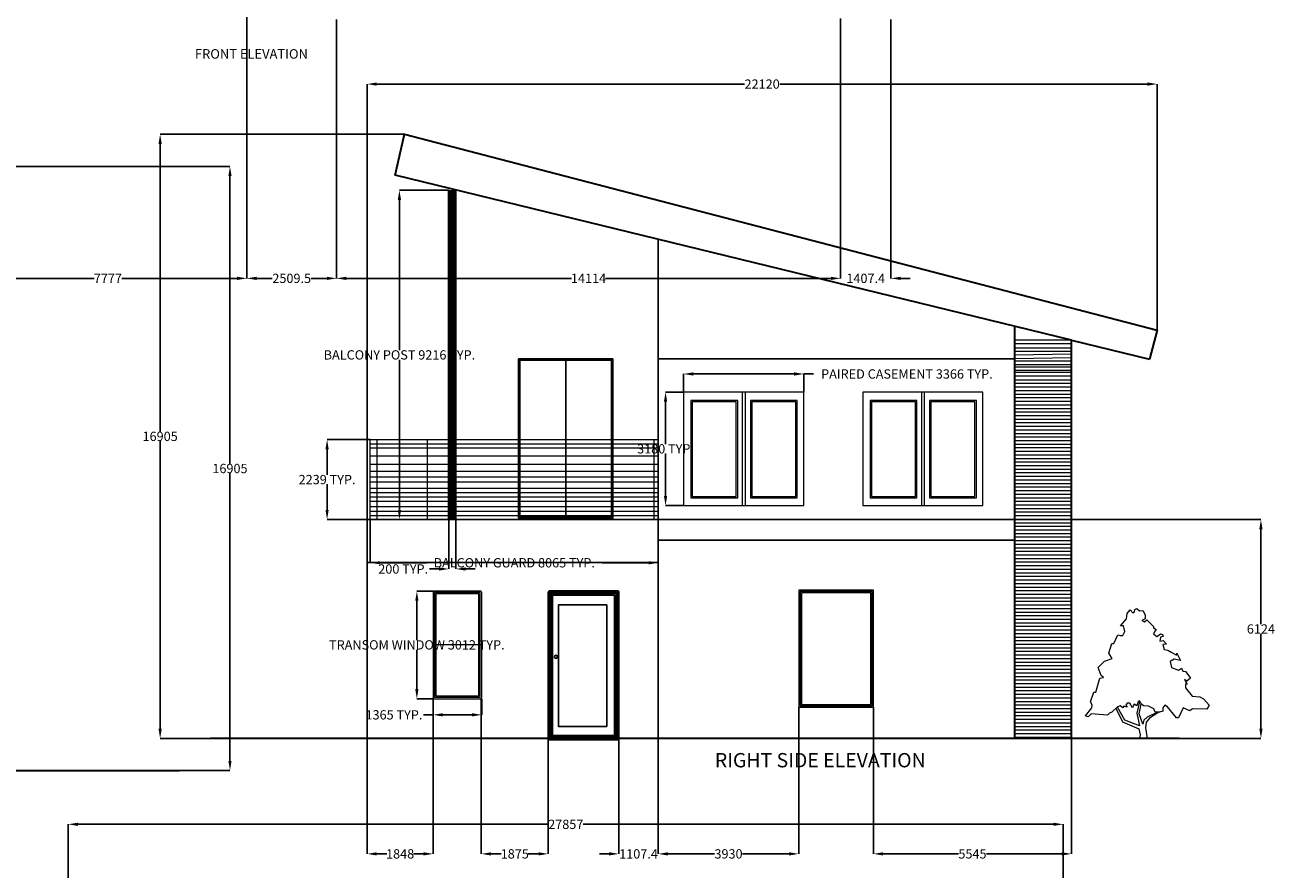
# Model space of a CAD drawing. Units: millimetres. Extents: x 23 to 3809233, y 4 to 290343.
# Tile 6 of 8: x 1915648 to 1950647, y 149481 to 173128. Entities that reach past the tile are written whole.
import ezdxf

# ---------------------------------------------------------------- set-up
doc = ezdxf.new("R2010")
doc.units = ezdxf.units.MM
doc.header["$MEASUREMENT"] = 0
for name, color, linetype, lineweight in [('A-ANNO-DIMS', 2, 'Continuous', 18), ('A-ANNO-TEXT', 7, 'Continuous', 25), ('A-COLS', 7, 'Continuous', 35), ('A-DOOR', 3, 'Continuous', 25), ('A-ELEV', 7, 'Continuous', 25), ('A-ELEV-GRND', 7, 'Continuous', 30), ('A-FLOR-RAIL', 8, 'Continuous', 18), ('A-GLAZ', 4, 'Continuous', 18), ('A-ROOF', 7, 'Continuous', 35), ('A-WALL-PATT', 252, 'Continuous', 13), ('L-PLNT', 94, 'Continuous', 13)]:
    doc.layers.add(name, color=color, linetype=linetype, lineweight=lineweight)
doc.styles.get("Standard").update_dxf_attribs({"font": 'arial.ttf'})
doc.dimstyles.get("Standard").update_dxf_attribs({"dimtxt": 260.18, "dimasz": 270.18, "dimexe": 0.18, "dimexo": 0.0625, "dimgap": 0.09, "dimtad": 0, "dimtih": 1, "dimtoh": 1, "dimdec": 0, "dimzin": 0, "dimdsep": 46, "dimtxsty": 'Standard', "dimcen": 0.09, "dimadec": 0, "dimazin": 0, "dimtfac": 1, "dimtdec": 0, "dimtofl": 0, "dimtmove": 0, "dimatfit": 3, "dimfxl": 1, "dimtolj": 1, "dimtzin": 0, "dimarcsym": 0})

# ---------------------------------------------------------------- blocks, each defined once
blk = doc.blocks.new('*U4')
for points in [[(22.0124, 137.721), (18.5475, 141.5624), (15.5282, 138.2446), (13.8028, 139.3505), (13.3714, 142.1153), (11.2148, 143.2214), (8.1954, 140.4564), (4.7447, 141.0094), (2.1567, 136.0326), (2.1567, 131.6088), (5.6074, 129.9499), (3.0193, 128.2909), (0.4313, 130.5029), (-6.9015, 123.3141), (-6.9015, 121.6552), (-9.9208, 119.9963), (-9.0581, 118.3373), (-6.9015, 115.0195), (-10.7835, 112.2546), (-14.6656, 115.0195), (-16.8222, 114.4665), (-17.6849, 112.2546), (-14.6656, 111.7016), (-14.2342, 107.2778), (-17.6065, 107.8307), (-21.5669, 103.9599), (-17.2536, 103.4069), (-18.9789, 97.8771), (-22.8609, 97.3241), (-27.1743, 94.5593), (-32.3504, 91.7944), (-32.7817, 94.0063), (-36.6638, 85.7116), (-29.7624, 87.3705), (-25.449, 84.6056), (-26.743, 77.9699), (-34.507, 75.205), (-37.9578, 77.4169), (-39.2518, 74.099), (-42.2711, 73.5461), (-44.8592, 70.2282), (-47.8786, 66.3574), (-43.9965, 63.0395), (-41.4085, 64.6985), (-44.3346, 59.8898), (-42.2089, 60.1377), (-42.5159, 55.7849), (-49.6039, 46.4502), (-58.2307, 45.8972), (-62.1127, 43.6853), (-68.5828, 36.4966), (-65.9947, 32.0727), (-50.0352, 32.6257), (-47.0159, 30.4138), (-39.6831, 33.7317), (-34.507, 22.6721), (-32.3504, 22.6721), (-22.4296, 34.8376), (-19.4102, 36.4966), (-17.2536, 33.7317), (-17.2536, 29.8608), (-13.8028, 28.7549), (-9.0581, 28.7549), (-7.3328, 32.6257), (-1.7254, 35.3906), (3.8821, 35.9436), (6.4701, 38.1555), (6.9014, 38.7085), (8.1954, 41.4734), (9.9208, 40.3674), (11.2148, 35.9436), (14.2341, 37.6025), (15.0968, 36.4966), (15.9595, 33.7317), (18.9789, 38.7085), (21.9982, 38.7085), (23.2922, 36.4966), (21.9982, 34.2847), (25.4489, 35.3906), (26.743, 33.7317), (29.7623, 35.9436), (32.7817, 34.8376), (38.8204, 28.7549), (41.4084, 27.6489), (43.5651, 25.437), (61.6813, 27.0959), (65.132, 23.7781), (67.7201, 24.884), (60.8186, 33.7317), (60.3873, 37.0495), (62.544, 40.3674), (58.662, 50.874), (56.5053, 50.874), (52.1919, 66.3574), (47.8785, 66.9103), (50.4665, 69.1222), (53.9172, 77.9699), (47.0158, 85.1586), (38.3891, 87.9235), (42.2711, 94.0063)], [(42.2711, 94.0063), (38.8204, 104.5129), (36.6637, 104.5129), (32.3503, 113.9135), (29.7623, 113.3605), (26.743, 113.3605), (24.5862, 117.7844), (25.8802, 123.8671), (29.331, 123.8671), (22.8609, 131.6088), (21.9982, 137.6916)], [(-12.9401, 28.7549), (-2.588, 22.1191), (0.8626, 17.6953), (1.7253, 11.6125), (0, 0)], [(-9.9208, 28.2019), (0, 23.2251), (3.4507, 19.9072), (4.7447, 15.4834), (8.6267, 27.0959), (6.4701, 37.6025)], [(34.5071, 33.1787), (27.1743, 18.2483), (9.0581, 10.5066), (7.7641, 3.8708), (8.1954, 0)], [(8.1954, 40.3674), (11.2148, 27.6489), (8.1954, 13.8245), (24.5862, 19.9072), (32.7817, 34.2847)]]:
    blk.add_lwpolyline(points)
blk = doc.blocks.new('SIDE-ENTRY-DOOR-ELEV')
for points in [[(0, 4129, -0.414214), (43, 4172), (1935, 4172, -0.414214), (1978, 4129), (1978, 43, -0.414214), (1935, 0), (43, 0, -0.414214), (0, 43)], [(40, 4129, -0.414214), (43, 4132), (1935, 4132, -0.414214), (1938, 4129), (1938, 43, -0.414214), (1935, 40), (43, 40, -0.414214), (40, 43)], [(337, 3772, -0.414214), (340, 3775), (1691, 3775, -0.414214), (1694, 3772), (1694, 380, -0.414214), (1691, 377), (340, 377, -0.414214), (337, 380)]]:
    blk.add_lwpolyline(points, format="xyb", close=True)
for points in [[(80, 4092), (1898, 4092), (1898, 80), (80, 80)], [(120, 4052), (1858, 4052), (1858, 120), (120, 120)]]:
    blk.add_lwpolyline(points, close=True)
blk.add_circle((1762, 2322), 43.3)
blk = doc.blocks.new('FIXED-WINDOW-ELEV')
blk.add_lwpolyline([(0, 3279, -0.414214), (3, 3282), (2093, 3282, -0.414214), (2096, 3279), (2096, 3, -0.414214), (2093, 0), (3, 0, -0.414214), (0, 3)], format="xyb", close=True)
for points in [[(40, 3242), (2056, 3242), (2056, 40), (40, 40)], [(80, 3202), (2016, 3202), (2016, 80), (80, 80)]]:
    blk.add_lwpolyline(points, close=True)
blk = doc.blocks.new('TRANSOM-WINDOW-ELEV')
blk.add_line((0, 1506), (1365, 1506))
for points in [[(0, 2969, -0.414214), (43, 3012), (1322, 3012, -0.414214), (1365, 2969), (1365, 43, -0.414214), (1322, 0), (43, 0, -0.414214), (0, 43)], [(40, 2969, -0.414214), (43, 2972), (1322, 2972, -0.414214), (1325, 2969), (1325, 43, -0.414214), (1322, 40), (43, 40, -0.414214), (40, 43)]]:
    blk.add_lwpolyline(points, format="xyb", close=True)
blk.add_lwpolyline([(80, 2932), (1285, 2932), (1285, 80), (80, 80)], close=True)
blk = doc.blocks.new('BALCONY-GUARD-ELEV')
for p, q in [((8065, 2239), (0, 2239)), ((0, 2109), (8065, 2109)), ((129, 2239), (129, 0)), ((6472, 2239), (6472, 0)), ((7879, 2239), (7879, 0)), ((8065, 0), (8065, 2239)), ((0, 1995), (8065, 1995)), ((0, 1772), (8065, 1772)), ((0, 1540), (8065, 1540)), ((0, 1341), (8065, 1341)), ((0, 1187), (8065, 1187)), ((0, 1045), (8065, 1045)), ((0, 866), (8065, 866)), ((0, 745), (8065, 745)), ((0, 622), (8065, 622)), ((0, 507), (8065, 507)), ((0, 360), (8065, 360)), ((8065, 360), (8065, 360)), ((0, 225), (8065, 225)), ((0, 103), (8065, 103))]:
    blk.add_line(p, q)
blk = doc.blocks.new('PAIRED-CASEMENT-ELEV')
for p, q in [((1643, 3180), (1643, 0)), ((1723, 3180), (1723, 0))]:
    blk.add_line(p, q)
for points in [[(3366, 3177, 0.414214), (3363, 3180), (3, 3180, 0.414214), (0, 3177), (0, 3, 0.414214), (3, 0), (3363, 0, 0.414214), (3366, 3)], [(1515, 2942, 0.414214), (1512, 2945), (206, 2945, 0.414214), (203, 2942), (203, 222, 0.414214), (206, 219), (1512, 219, 0.414214), (1515, 222)], [(3181, 2942, 0.414214), (3178, 2945), (1873, 2945, 0.414214), (1870, 2942), (1870, 222, 0.414214), (1873, 219), (3178, 219, 0.414214), (3181, 222)]]:
    blk.add_lwpolyline(points, format="xyb", close=True)
for points in [[(1475, 2905), (243, 2905), (243, 259), (1475, 259)], [(3141, 2905), (1910, 2905), (1910, 259), (3141, 259)]]:
    blk.add_lwpolyline(points, close=True)
blk = doc.blocks.new('ROOF-FASCIA-SIDE-ELEV')
for p, q in [((21076, 6297), (0, 817)), ((21331, 5154), (21076, 6297)), ((2399, 534), (21331, 5154)), ((0, 817), (212, 0)), ((2399, 534), (212, 0))]:
    blk.add_line(p, q)
blk = doc.blocks.new('BALCONY-SUPPORT-ELEV')
for p, q in [((0, 0), (0, 9216)), ((40, 0), (40, 9216)), ((80, 0), (80, 9216)), ((120, 0), (120, 9216)), ((120, 0), (120, 9216)), ((160, 0), (160, 9216)), ((200, 0), (200, 9216))]:
    blk.add_line(p, q)
blk = doc.blocks.new('BALCONY-GLAZED-DOOR-ELEV')
for p, q in [((0, 4461), (2642, 4461)), ((0, 4421), (2642, 4421)), ((1321, 4461), (1321, 0))]:
    blk.add_line(p, q)
for points in [[(0, 4461), (0, 0), (2642, 0), (2642, 4461)], [(40, 4461), (40, 40), (2602, 40), (2602, 4461)]]:
    blk.add_lwpolyline(points)
blk = doc.blocks.new('*D30')
at = {"layer": 'A-ANNO-DIMS', "color": 0, "lineweight": -2, "transparency": 16777216}
for p, q in [((1927514, 168504), (1926131, 168504)), ((1926132, 168234), (1926132, 164031)), ((1926132, 159558), (1926132, 163761)), ((1927514, 159288), (1926131, 159288))]:
    blk.add_line(p, q, dxfattribs=at)
at = {"layer": 'A-ANNO-DIMS', "color": 0, "transparency": 16777216}
for points in [[(1926087, 168234), (1926177, 168234), (1926132, 168504)], [(1926087, 159558), (1926177, 159558), (1926132, 159288)]]:
    blk.add_solid(points, dxfattribs=at)
at = {"layer": 'Defpoints', "color": 0, "transparency": 16777216}
for p in [(1926132, 168504), (1927514, 168504), (1927514, 159288)]:
    blk.add_point(p, dxfattribs=at)
at = {"layer": 'A-ANNO-DIMS', "color": 0, "transparency": 16777216, "insert": (1926132, 163896), "char_height": 260.18, "attachment_point": 5}
blk.add_mtext('\\A1;BALCONY POST 9216 TYP.', dxfattribs=at)
blk = doc.blocks.new('*D31')
at = {"layer": 'A-ANNO-DIMS', "color": 0, "lineweight": -2, "transparency": 16777216}
for p, q in [((1927514, 159288), (1927514, 157905)), ((1927714, 159288), (1927714, 157905)), ((1927244, 157905), (1926974, 157905)), ((1927984, 157905), (1928254, 157905))]:
    blk.add_line(p, q, dxfattribs=at)
at = {"layer": 'A-ANNO-DIMS', "color": 0, "transparency": 16777216}
for points in [[(1927244, 157950), (1927244, 157860), (1927514, 157905)], [(1927984, 157950), (1927984, 157860), (1927714, 157905)]]:
    blk.add_solid(points, dxfattribs=at)
at = {"layer": 'Defpoints', "color": 0, "transparency": 16777216}
for p in [(1927514, 159288), (1927714, 159288), (1927514, 157905)]:
    blk.add_point(p, dxfattribs=at)
at = {"layer": 'A-ANNO-DIMS', "color": 0, "transparency": 16777216, "insert": (1926237, 157905), "char_height": 260.18, "attachment_point": 5}
blk.add_mtext('\\A1;200 TYP.', dxfattribs=at)
blk = doc.blocks.new('*D38')
at = {"layer": 'A-ANNO-DIMS', "color": 0, "lineweight": -2, "transparency": 16777216}
for p, q in [((1927072, 157287), (1926620, 157287)), ((1926620, 157017), (1926620, 155916)), ((1926620, 154545), (1926620, 155646)), ((1927072, 154275), (1926620, 154275))]:
    blk.add_line(p, q, dxfattribs=at)
at = {"layer": 'A-ANNO-DIMS', "color": 0, "transparency": 16777216}
for points in [[(1926575, 157017), (1926665, 157017), (1926620, 157287)], [(1926575, 154545), (1926665, 154545), (1926620, 154275)]]:
    blk.add_solid(points, dxfattribs=at)
at = {"layer": 'Defpoints', "color": 0, "transparency": 16777216}
for p in [(1926620, 157287), (1927072, 157287), (1927072, 154275)]:
    blk.add_point(p, dxfattribs=at)
at = {"layer": 'A-ANNO-DIMS', "color": 0, "transparency": 16777216, "insert": (1926620, 155781), "char_height": 260.18, "attachment_point": 5}
blk.add_mtext('\\A1;TRANSOM WINDOW 3012 TYP.', dxfattribs=at)
blk = doc.blocks.new('*D39')
at = {"layer": 'A-ANNO-DIMS', "color": 0, "lineweight": -2, "transparency": 16777216}
for p, q in [((1927072, 154275), (1927072, 153823)), ((1928437, 154275), (1928437, 153823)), ((1927072, 153823), (1926802, 153823)), ((1928167, 153823), (1927342, 153823))]:
    blk.add_line(p, q, dxfattribs=at)
at = {"layer": 'A-ANNO-DIMS', "color": 0, "transparency": 16777216}
for points in [[(1927342, 153868), (1927342, 153778), (1927072, 153823)], [(1928167, 153868), (1928167, 153778), (1928437, 153823)]]:
    blk.add_solid(points, dxfattribs=at)
at = {"layer": 'Defpoints', "color": 0, "transparency": 16777216}
for p in [(1927072, 154275), (1928437, 154275), (1927072, 153823)]:
    blk.add_point(p, dxfattribs=at)
at = {"layer": 'A-ANNO-DIMS', "color": 0, "transparency": 16777216, "insert": (1925978, 153823), "char_height": 260.18, "attachment_point": 5}
blk.add_mtext('\\A1;1365 TYP.', dxfattribs=at)
blk = doc.blocks.new('*D40')
at = {"layer": 'A-ANNO-DIMS', "color": 0, "lineweight": -2, "transparency": 16777216}
for p, q in [((1934088, 162857), (1934088, 163362)), ((1934358, 163362), (1937184, 163362)), ((1937454, 162857), (1937454, 163362)), ((1937454, 163362), (1937724, 163362))]:
    blk.add_line(p, q, dxfattribs=at)
at = {"layer": 'A-ANNO-DIMS', "color": 0, "transparency": 16777216}
for points in [[(1934358, 163407), (1934358, 163317), (1934088, 163362)], [(1937184, 163407), (1937184, 163317), (1937454, 163362)]]:
    blk.add_solid(points, dxfattribs=at)
at = {"layer": 'Defpoints', "color": 0, "transparency": 16777216}
for p in [(1937454, 163362), (1934088, 162857), (1937454, 162857)]:
    blk.add_point(p, dxfattribs=at)
at = {"layer": 'A-ANNO-DIMS', "color": 0, "transparency": 16777216, "insert": (1940341, 163362), "char_height": 260.18, "attachment_point": 5}
blk.add_mtext('\\A1;PAIRED CASEMENT 3366 TYP.', dxfattribs=at)
blk = doc.blocks.new('*D41')
at = {"layer": 'A-ANNO-DIMS', "color": 0, "lineweight": -2, "transparency": 16777216}
for p, q in [((1934088, 162857), (1933583, 162857)), ((1933583, 162587), (1933583, 161400)), ((1933583, 159947), (1933583, 161134)), ((1934088, 159677), (1933583, 159677))]:
    blk.add_line(p, q, dxfattribs=at)
at = {"layer": 'A-ANNO-DIMS', "color": 0, "transparency": 16777216}
for points in [[(1933538, 162587), (1933628, 162587), (1933583, 162857)], [(1933538, 159947), (1933628, 159947), (1933583, 159677)]]:
    blk.add_solid(points, dxfattribs=at)
at = {"layer": 'Defpoints', "color": 0, "transparency": 16777216}
for p in [(1933583, 162857), (1934088, 162857), (1934088, 159677)]:
    blk.add_point(p, dxfattribs=at)
at = {"layer": 'A-ANNO-DIMS', "color": 0, "transparency": 16777216, "insert": (1933583, 161267), "char_height": 260.18, "attachment_point": 5}
blk.add_mtext('\\A1;3180 TYP.', dxfattribs=at)
blk = doc.blocks.new('*D42')
at = {"layer": 'A-ANNO-DIMS', "color": 0, "lineweight": -2, "transparency": 16777216}
for p, q in [((1925316, 159288), (1925316, 158078)), ((1933381, 159288), (1933381, 158078)), ((1925586, 158078), (1926893, 158078)), ((1933111, 158078), (1931804, 158078))]:
    blk.add_line(p, q, dxfattribs=at)
at = {"layer": 'A-ANNO-DIMS', "color": 0, "transparency": 16777216}
for points in [[(1925586, 158123), (1925586, 158033), (1925316, 158078)], [(1933111, 158123), (1933111, 158033), (1933381, 158078)]]:
    blk.add_solid(points, dxfattribs=at)
at = {"layer": 'Defpoints', "color": 0, "transparency": 16777216}
for p in [(1925316, 159288), (1933381, 159288), (1925316, 158078)]:
    blk.add_point(p, dxfattribs=at)
at = {"layer": 'A-ANNO-DIMS', "color": 0, "transparency": 16777216, "insert": (1929348, 158078), "char_height": 260.18, "attachment_point": 5}
blk.add_mtext('\\A1;BALCONY GUARD 8065 TYP.', dxfattribs=at)
blk = doc.blocks.new('*D43')
at = {"layer": 'A-ANNO-DIMS', "color": 0, "lineweight": -2, "transparency": 16777216}
for p, q in [((1925316, 161527), (1924106, 161527)), ((1924106, 161257), (1924106, 160540)), ((1924106, 159558), (1924106, 160274)), ((1925316, 159288), (1924106, 159288))]:
    blk.add_line(p, q, dxfattribs=at)
at = {"layer": 'A-ANNO-DIMS', "color": 0, "transparency": 16777216}
for points in [[(1924061, 161257), (1924151, 161257), (1924106, 161527)], [(1924061, 159558), (1924151, 159558), (1924106, 159288)]]:
    blk.add_solid(points, dxfattribs=at)
at = {"layer": 'Defpoints', "color": 0, "transparency": 16777216}
for p in [(1924106, 161527), (1925316, 161527), (1925316, 159288)]:
    blk.add_point(p, dxfattribs=at)
at = {"layer": 'A-ANNO-DIMS', "color": 0, "transparency": 16777216, "insert": (1924106, 160407), "char_height": 260.18, "attachment_point": 5}
blk.add_mtext('\\A1;2239 TYP.', dxfattribs=at)
blk = doc.blocks.new('*D81')
at = {"layer": 'A-ANNO-DIMS', "color": 0, "lineweight": -2, "transparency": 16777216}
for p, q in [((1914545, 169170), (1921388, 169170)), ((1921387, 168900), (1921387, 160850)), ((1921387, 152535), (1921387, 160584)), ((1915588, 152265), (1921388, 152265))]:
    blk.add_line(p, q, dxfattribs=at)
at = {"layer": 'A-ANNO-DIMS', "color": 0, "transparency": 16777216}
for points in [[(1921342, 168900), (1921433, 168900), (1921387, 169170)], [(1921342, 152535), (1921433, 152535), (1921387, 152265)]]:
    blk.add_solid(points, dxfattribs=at)
at = {"layer": 'Defpoints', "color": 0, "transparency": 16777216}
for p in [(1914545, 169170), (1921387, 169170), (1915588, 152265)]:
    blk.add_point(p, dxfattribs=at)
at = {"layer": 'A-ANNO-DIMS', "color": 0, "transparency": 16777216, "insert": (1921387, 160717), "char_height": 260.2, "attachment_point": 5}
blk.add_mtext('\\A1;16905', dxfattribs=at)
blk = doc.blocks.new('*D86')
at = {"layer": 'A-ANNO-DIMS', "color": 0, "lineweight": -2, "transparency": 16777216}
for p, q in [((1925227, 153164), (1925227, 171475)), ((1925497, 171475), (1935796, 171475)), ((1947077, 171475), (1936779, 171475)), ((1947347, 164589), (1947347, 171475))]:
    blk.add_line(p, q, dxfattribs=at)
at = {"layer": 'A-ANNO-DIMS', "color": 0, "transparency": 16777216}
for points in [[(1925497, 171520), (1925497, 171430), (1925227, 171475)], [(1947077, 171520), (1947077, 171430), (1947347, 171475)]]:
    blk.add_solid(points, dxfattribs=at)
at = {"layer": 'Defpoints', "color": 0, "transparency": 16777216}
for p in [(1947347, 171475), (1947347, 164589), (1925227, 153164)]:
    blk.add_point(p, dxfattribs=at)
at = {"layer": 'A-ANNO-DIMS', "color": 0, "transparency": 16777216, "insert": (1936287, 171475), "char_height": 260.2, "attachment_point": 5}
blk.add_mtext('\\A1;22120', dxfattribs=at)
blk = doc.blocks.new('*D87')
at = {"layer": 'A-ANNO-DIMS', "color": 0, "lineweight": -2, "transparency": 16777216}
for p, q in [((1926271, 170069), (1919431, 170069)), ((1919432, 169799), (1919432, 161749)), ((1919432, 153434), (1919432, 161484)), ((1925227, 153164), (1919431, 153164))]:
    blk.add_line(p, q, dxfattribs=at)
at = {"layer": 'A-ANNO-DIMS', "color": 0, "transparency": 16777216}
for points in [[(1919387, 169799), (1919477, 169799), (1919432, 170069)], [(1919387, 153434), (1919477, 153434), (1919432, 153164)]]:
    blk.add_solid(points, dxfattribs=at)
at = {"layer": 'Defpoints', "color": 0, "transparency": 16777216}
for p in [(1919432, 170069), (1926271, 170069), (1925227, 153164)]:
    blk.add_point(p, dxfattribs=at)
at = {"layer": 'A-ANNO-DIMS', "color": 0, "transparency": 16777216, "insert": (1919432, 161616), "char_height": 260.2, "attachment_point": 5}
blk.add_mtext('\\A1;16905', dxfattribs=at)
blk = doc.blocks.new('*D88')
at = {"layer": 'A-ANNO-DIMS', "color": 0, "lineweight": -2, "transparency": 16777216}
for p, q in [((1927075, 154301), (1927075, 149932)), ((1925227, 153164), (1925227, 149932)), ((1925497, 149932), (1925775, 149932)), ((1926805, 149932), (1926528, 149932))]:
    blk.add_line(p, q, dxfattribs=at)
at = {"layer": 'A-ANNO-DIMS', "color": 0, "transparency": 16777216}
for points in [[(1925497, 149977), (1925497, 149887), (1925227, 149932)], [(1926805, 149977), (1926805, 149887), (1927075, 149932)]]:
    blk.add_solid(points, dxfattribs=at)
at = {"layer": 'Defpoints', "color": 0, "transparency": 16777216}
for p in [(1927075, 154301), (1925227, 153164), (1927075, 149932)]:
    blk.add_point(p, dxfattribs=at)
at = {"layer": 'A-ANNO-DIMS', "color": 0, "transparency": 16777216, "insert": (1926151, 149932), "char_height": 260.2, "attachment_point": 5}
blk.add_mtext('\\A1;1848', dxfattribs=at)
blk = doc.blocks.new('*D89')
at = {"layer": 'A-ANNO-DIMS', "color": 0, "lineweight": -2, "transparency": 16777216}
for p, q in [((1928425, 154288), (1928425, 149932)), ((1930299, 153167), (1930299, 149932)), ((1928695, 149932), (1928985, 149932)), ((1930029, 149932), (1929739, 149932))]:
    blk.add_line(p, q, dxfattribs=at)
at = {"layer": 'A-ANNO-DIMS', "color": 0, "transparency": 16777216}
for points in [[(1928695, 149977), (1928695, 149887), (1928425, 149932)], [(1930029, 149977), (1930029, 149887), (1930299, 149932)]]:
    blk.add_solid(points, dxfattribs=at)
at = {"layer": 'Defpoints', "color": 0, "transparency": 16777216}
for p in [(1928425, 154288), (1930299, 153167), (1930299, 149932)]:
    blk.add_point(p, dxfattribs=at)
at = {"layer": 'A-ANNO-DIMS', "color": 0, "transparency": 16777216, "insert": (1929362, 149932), "char_height": 260.2, "attachment_point": 5}
blk.add_mtext('\\A1;1875', dxfattribs=at)
blk = doc.blocks.new('*D90')
at = {"layer": 'A-ANNO-DIMS', "color": 0, "lineweight": -2, "transparency": 16777216}
for p, q in [((1932274, 153150), (1932274, 149932)), ((1933381, 153164), (1933381, 149932)), ((1932003, 149932), (1931733, 149932)), ((1933651, 149932), (1933921, 149932))]:
    blk.add_line(p, q, dxfattribs=at)
at = {"layer": 'A-ANNO-DIMS', "color": 0, "transparency": 16777216}
for points in [[(1932003, 149977), (1932003, 149887), (1932274, 149932)], [(1933651, 149977), (1933651, 149887), (1933381, 149932)]]:
    blk.add_solid(points, dxfattribs=at)
at = {"layer": 'Defpoints', "color": 0, "transparency": 16777216}
for p in [(1932274, 153150), (1933381, 153164), (1933381, 149932)]:
    blk.add_point(p, dxfattribs=at)
at = {"layer": 'A-ANNO-DIMS', "color": 0, "transparency": 16777216, "insert": (1932827, 149932), "char_height": 260.2, "attachment_point": 5}
blk.add_mtext('\\A1;1107.4', dxfattribs=at)
blk = doc.blocks.new('*D91')
at = {"layer": 'A-ANNO-DIMS', "color": 0, "lineweight": -2, "transparency": 16777216}
for p, q in [((1937311, 154036), (1937311, 149932)), ((1933381, 153164), (1933381, 149932)), ((1933651, 149932), (1934958, 149932)), ((1937041, 149932), (1935734, 149932))]:
    blk.add_line(p, q, dxfattribs=at)
at = {"layer": 'A-ANNO-DIMS', "color": 0, "transparency": 16777216}
for points in [[(1933651, 149977), (1933651, 149887), (1933381, 149932)], [(1937041, 149977), (1937041, 149887), (1937311, 149932)]]:
    blk.add_solid(points, dxfattribs=at)
at = {"layer": 'Defpoints', "color": 0, "transparency": 16777216}
for p in [(1937311, 154036), (1933381, 153164), (1937311, 149932)]:
    blk.add_point(p, dxfattribs=at)
at = {"layer": 'A-ANNO-DIMS', "color": 0, "transparency": 16777216, "insert": (1935346, 149932), "char_height": 260.2, "attachment_point": 5}
blk.add_mtext('\\A1;3930', dxfattribs=at)
blk = doc.blocks.new('*D92')
at = {"layer": 'A-ANNO-DIMS', "color": 0, "lineweight": -2, "transparency": 16777216}
for p, q in [((1939403, 154033), (1939403, 149932)), ((1944948, 153164), (1944948, 149932)), ((1939674, 149932), (1941786, 149932)), ((1944678, 149932), (1942565, 149932))]:
    blk.add_line(p, q, dxfattribs=at)
at = {"layer": 'A-ANNO-DIMS', "color": 0, "transparency": 16777216}
for points in [[(1939674, 149977), (1939674, 149887), (1939403, 149932)], [(1944678, 149977), (1944678, 149887), (1944948, 149932)]]:
    blk.add_solid(points, dxfattribs=at)
at = {"layer": 'Defpoints', "color": 0, "transparency": 16777216}
for p in [(1939403, 154033), (1944948, 153164), (1944948, 149932)]:
    blk.add_point(p, dxfattribs=at)
at = {"layer": 'A-ANNO-DIMS', "color": 0, "transparency": 16777216, "insert": (1942176, 149932), "char_height": 260.2, "attachment_point": 5}
blk.add_mtext('\\A1;5545', dxfattribs=at)
blk = doc.blocks.new('*D93')
at = {"layer": 'A-ANNO-DIMS', "color": 0, "lineweight": -2, "transparency": 16777216}
for p, q in [((1933379, 159288), (1950253, 159288)), ((1950253, 159017), (1950253, 156359)), ((1950253, 153434), (1950253, 156093)), ((1944948, 153164), (1950253, 153164))]:
    blk.add_line(p, q, dxfattribs=at)
at = {"layer": 'A-ANNO-DIMS', "color": 0, "transparency": 16777216}
for points in [[(1950208, 159017), (1950298, 159017), (1950253, 159288)], [(1950208, 153434), (1950298, 153434), (1950253, 153164)]]:
    blk.add_solid(points, dxfattribs=at)
at = {"layer": 'Defpoints', "color": 0, "transparency": 16777216}
for p in [(1933379, 159288), (1950253, 159288), (1944948, 153164)]:
    blk.add_point(p, dxfattribs=at)
at = {"layer": 'A-ANNO-DIMS', "color": 0, "transparency": 16777216, "insert": (1950253, 156226), "char_height": 260.2, "attachment_point": 5}
blk.add_mtext('\\A1;6124', dxfattribs=at)
blk = doc.blocks.new('*D99')
at = {"layer": 'A-ANNO-DIMS', "color": 0, "lineweight": -2, "transparency": 16777216}
for p, q in [((1921861, 173281), (1921861, 166038)), ((1924370, 173282), (1924370, 166038)), ((1922131, 166038), (1922572, 166038)), ((1924100, 166038), (1923659, 166038))]:
    blk.add_line(p, q, dxfattribs=at)
at = {"layer": 'A-ANNO-DIMS', "color": 0, "transparency": 16777216}
for points in [[(1922131, 166083), (1922131, 165993), (1921861, 166038)], [(1924100, 166083), (1924100, 165993), (1924370, 166038)]]:
    blk.add_solid(points, dxfattribs=at)
at = {"layer": 'Defpoints', "color": 0, "transparency": 16777216}
for p in [(1921861, 173281), (1924370, 173282), (1924370, 166038)]:
    blk.add_point(p, dxfattribs=at)
at = {"layer": 'A-ANNO-DIMS', "color": 0, "transparency": 16777216, "insert": (1923116, 166038), "char_height": 260.2, "attachment_point": 5}
blk.add_mtext('\\A1;2509.5', dxfattribs=at)
blk = doc.blocks.new('*D100')
at = {"layer": 'A-ANNO-DIMS', "color": 0, "lineweight": -2, "transparency": 16777216}
for p, q in [((1924370, 173282), (1924370, 166038)), ((1938484, 173307), (1938484, 166038)), ((1924641, 166038), (1930950, 166038)), ((1938214, 166038), (1931904, 166038))]:
    blk.add_line(p, q, dxfattribs=at)
at = {"layer": 'A-ANNO-DIMS', "color": 0, "transparency": 16777216}
for points in [[(1924641, 166083), (1924641, 165993), (1924370, 166038)], [(1938214, 166083), (1938214, 165993), (1938484, 166038)]]:
    blk.add_solid(points, dxfattribs=at)
at = {"layer": 'Defpoints', "color": 0, "transparency": 16777216}
for p in [(1924370, 173282), (1938484, 173307), (1938484, 166038)]:
    blk.add_point(p, dxfattribs=at)
at = {"layer": 'A-ANNO-DIMS', "color": 0, "transparency": 16777216, "insert": (1931427, 166038), "char_height": 260.2, "attachment_point": 5}
blk.add_mtext('\\A1;14114', dxfattribs=at)
blk = doc.blocks.new('*D101')
at = {"layer": 'A-ANNO-DIMS', "color": 0, "lineweight": -2, "transparency": 16777216}
for p, q in [((1938484, 173307), (1938484, 166038)), ((1939891, 173281), (1939891, 166038)), ((1938214, 166038), (1937944, 166038)), ((1940162, 166038), (1940432, 166038))]:
    blk.add_line(p, q, dxfattribs=at)
at = {"layer": 'A-ANNO-DIMS', "color": 0, "transparency": 16777216}
for points in [[(1938214, 166083), (1938214, 165993), (1938484, 166038)], [(1940162, 166083), (1940162, 165993), (1939891, 166038)]]:
    blk.add_solid(points, dxfattribs=at)
at = {"layer": 'Defpoints', "color": 0, "transparency": 16777216}
for p in [(1938484, 173307), (1939891, 173281), (1939891, 166038)]:
    blk.add_point(p, dxfattribs=at)
at = {"layer": 'A-ANNO-DIMS', "color": 0, "transparency": 16777216, "insert": (1939188, 166038), "char_height": 260.2, "attachment_point": 5}
blk.add_mtext('\\A1;1407.4', dxfattribs=at)
blk = doc.blocks.new('*D102')
at = {"layer": 'A-ANNO-DIMS', "color": 0, "lineweight": -2, "transparency": 16777216}
for p, q in [((1914079.851314, 175025.824019), (1914079.851314, 166037.51032)), ((1921856.95103, 175025.824019), (1921856.95103, 166037.51032)), ((1914350.031314, 166037.69032), (1917580.88079, 166037.69032)), ((1921586.77103, 166037.69032), (1918355.921554, 166037.69032))]:
    blk.add_line(p, q, dxfattribs=at)
at = {"layer": 'A-ANNO-DIMS', "color": 0, "transparency": 16777216}
for points in [[(1914350.031314, 166082.72032), (1914350.031314, 165992.66032), (1914079.851314, 166037.69032)], [(1921586.77103, 166082.72032), (1921586.77103, 165992.66032), (1921856.95103, 166037.69032)]]:
    blk.add_solid(points, dxfattribs=at)
at = {"layer": 'Defpoints', "color": 0, "transparency": 16777216}
for p in [(1914079.851314, 175025.886519), (1921856.95103, 175025.886519), (1921856.95103, 166037.69032)]:
    blk.add_point(p, dxfattribs=at)
at = {"layer": 'A-ANNO-DIMS', "color": 0, "transparency": 16777216, "insert": (1917968.401172, 166037.69032), "char_height": 260.18, "attachment_point": 5}
blk.add_mtext('\\A1;7777', dxfattribs=at)
blk = doc.blocks.new('*D116')
at = {"layer": 'A-ANNO-DIMS', "color": 0, "lineweight": -2, "transparency": 16777216}
for p, q in [((1916860, 145073), (1916860, 150759)), ((1917130, 150759), (1930297, 150759)), ((1944447, 150759), (1931281, 150759)), ((1944717, 145084), (1944717, 150759))]:
    blk.add_line(p, q, dxfattribs=at)
at = {"layer": 'A-ANNO-DIMS', "color": 0, "transparency": 16777216}
for points in [[(1917130, 150804), (1917130, 150714), (1916860, 150759)], [(1944447, 150804), (1944447, 150714), (1944717, 150759)]]:
    blk.add_solid(points, dxfattribs=at)
at = {"layer": 'Defpoints', "color": 0, "transparency": 16777216}
for p in [(1944717, 150759), (1916860, 145073), (1944717, 145084)]:
    blk.add_point(p, dxfattribs=at)
at = {"layer": 'A-ANNO-DIMS', "color": 0, "transparency": 16777216, "insert": (1930789, 150759), "char_height": 260.2, "attachment_point": 5}
blk.add_mtext('\\A1;27857', dxfattribs=at)

msp = doc.modelspace()

# ---------------------------------------------------------------- hatches: boundary and pattern name
at = {"layer": 'A-WALL-PATT'}
h = msp.add_hatch(dxfattribs=at)
h.set_pattern_fill('ANSI31', color=256, scale=800, angle=-45, style=0)
h.paths.add_polyline_path([(1943359.736, 153163.774), (1944948.196, 153163.774), (1944948.196, 163269.193), (1943359.736, 163269.193)])

# ---------------------------------------------------------------- linework, layer by layer
at = {"layer": 'A-COLS'}
for p, q in [((1943359.736, 153163.774), (1943359.736, 164693.542)), ((1944948.196, 153163.774), (1944948.196, 164305.856))]:
    msp.add_line(p, q, dxfattribs=at)
at = {"layer": 'A-DOOR'}
msp.add_lwpolyline([(1932148.447, 159290.791, -0.414213562), (1932145.447, 159287.791), (1929429.621, 159287.791, -0.414213562), (1929426.621, 159290.791)], format="xyb", dxfattribs=at)
at = {"layer": 'A-ELEV'}
for p, q in [((1933380.948, 158706.938), (1933380.948, 167129.008)), ((1943359.736, 163790.273), (1933380.948, 163790.273)), ((1925227.072, 153163.774), (1925227.072, 159284.791)), ((1943359.736, 158706.938), (1933380.948, 158706.938)), ((1933380.948, 158706.938), (1933380.948, 153163.774))]:
    msp.add_line(p, q, dxfattribs=at)
msp.add_lwpolyline([(1933380.948, 158091.878, -0.414213562), (1933377.948, 158088.878), (1925230.072, 158088.878, -0.414213562), (1925227.072, 158091.878), (1925227.072, 159284.791, -0.414213562), (1925230.072, 159287.791), (1933377.948, 159287.791, -0.414213562), (1933380.948, 159284.791)], format="xyb", close=True, dxfattribs=at)
at = {"layer": 'A-ELEV-GRND'}
for p, q in [((1947965.583, 153163.774), (1920837.416, 153163.774)), ((1892849.81, 152264.531), (1919977.977, 152264.531))]:
    msp.add_line(p, q, dxfattribs=at)
at = {"layer": 'A-WALL-PATT'}
for p, q in [((1944948.196, 164303.402), (1943359.736, 164303.402)), ((1944948.196, 164203.402), (1943359.736, 164203.402)), ((1944946.851, 163911.624), (1943358.391, 163890.264)), ((1944948.196, 164088.251), (1943359.736, 164088.251)), ((1944948.196, 163988.251), (1943359.736, 163988.251)), ((1944948.196, 163811.633), (1943359.736, 163790.273)), ((1944948.196, 163719.473), (1943359.736, 163719.473)), ((1944948.196, 163619.473), (1943359.736, 163619.473)), ((1944948.196, 163556.494), (1943359.736, 163556.494)), ((1944948.196, 163456.494), (1943359.736, 163456.494)), ((1944948.196, 163401.402), (1943359.736, 163401.402)), ((1944948.196, 163301.402), (1943359.736, 163301.402))]:
    msp.add_line(p, q, dxfattribs=at)

# ---------------------------------------------------------------- block references
at = {"layer": 'A-COLS', "extrusion": (0, 0, -1), "zscale": -1}
msp.add_blockref('BALCONY-SUPPORT-ELEV', (-1927714.03, 159287.791), dxfattribs=at)
at = {"layer": 'A-DOOR', "extrusion": (0, 0, -1), "zscale": -1}
for name, p in [('BALCONY-GLAZED-DOOR-ELEV', (-1932108.446, 159327.791)), ('SIDE-ENTRY-DOOR-ELEV', (-1932276.949, 153123.774))]:
    msp.add_blockref(name, p, dxfattribs=at)
at = {"layer": 'A-FLOR-RAIL', "extrusion": (0, 0, -1), "zscale": -1}
msp.add_blockref('BALCONY-GUARD-ELEV', (-1933380.947, 159287.791), dxfattribs=at)
at = {"layer": 'A-GLAZ'}
for p in [(1934088.053, 159677.011), (1939105.316, 159677.011)]:
    msp.add_blockref('PAIRED-CASEMENT-ELEV', p, dxfattribs=at)
at = {"layer": 'A-GLAZ', "extrusion": (0, 0, -1), "zscale": -1}
for name, p in [('TRANSOM-WINDOW-ELEV', (-1928437.159, 154275.054)), ('FIXED-WINDOW-ELEV', (-1939406.448, 154033.019))]:
    msp.add_blockref(name, p, dxfattribs=at)
at = {"layer": 'A-ROOF', "extrusion": (0, 0, -1), "zscale": -1}
msp.add_blockref('ROOF-FASCIA-SIDE-ELEV', (-1947347.07, 163772.22), dxfattribs=at)
at = {"layer": 'L-PLNT', "xscale": -25.4, "yscale": 25.4, "zscale": 25.4}
msp.add_blockref('*U4', (1947065.627, 153163.774), dxfattribs=at)

# ---------------------------------------------------------------- texts
at = {"layer": 'A-ANNO-TEXT', "attachment_point": 1}
for s, width, gutter_width, heights, insert, char_height in [('FRONT ELEVATION', 5579.04505, 0.663, [203.948], (1920407.063, 172452.25), 265.32835), ('RIGHT SIDE ELEVATION', 8410.77875, 1, [307.465], (1934963.262, 152753.389), 400)]:
    msp.add_mtext_dynamic_manual_height_columns(s, width=width, gutter_width=gutter_width, heights=heights, dxfattribs=dict(at, insert=insert, char_height=char_height))

# ---------------------------------------------------------------- dimensions: what is measured, and where the dimension line sits
at = {"layer": 'A-ANNO-DIMS'}
for base, p1, p2, override, picture, middle in [((1921856.951, 166037.69), (1914079.851, 175025.887), (1921856.951, 175025.887), {"dimdec": 0, "dimlfac": 1, "dimrnd": 0, "dimzin": 0, "dimdsep": 46, "dimlunit": 2}, '*D102', (1917968.401, 166037.69)), ((1924370.409, 166037.69), (1921860.931, 173280.749), (1924370.409, 173282.349), {"dimdec": 1, "dimlfac": 1, "dimrnd": 0, "dimzin": 0, "dimdsep": 46, "dimlunit": 2}, '*D99', (1923115.67, 166037.69)), ((1938483.986, 166037.69), (1924370.409, 173282.349), (1938483.986, 173307.282), {"dimdec": 0, "dimlfac": 1, "dimrnd": 0, "dimzin": 0, "dimdsep": 46, "dimlunit": 2}, '*D100', (1931427.197, 166037.69)), ((1939891.392, 166037.69), (1938483.986, 173307.282), (1939891.392, 173280.749), {"dimdec": 1, "dimlfac": 1, "dimrnd": 0, "dimzin": 0, "dimdsep": 46, "dimlunit": 2}, '*D101', (1939187.689, 166037.69)), ((1947347.07, 171474.893), (1925227.072, 153163.774), (1947347.07, 164589.214), {"dimdec": 0, "dimlfac": 1, "dimrnd": 0, "dimzin": 0, "dimdsep": 46, "dimlunit": 2}, '*D86', (1936287.071, 171474.893)), ((1927075.235, 149932.094), (1925227.072, 153163.774), (1927075.235, 154301.317), {"dimdec": 0, "dimlfac": 1, "dimrnd": 0, "dimzin": 0, "dimdsep": 46, "dimlunit": 2}, '*D88', (1926151.153, 149932.094)), ((1930299.443, 149932.094), (1928424.565, 154287.649), (1930299.443, 153166.774), {"dimdec": 0, "dimlfac": 1, "dimrnd": 0, "dimzin": 0, "dimdsep": 46, "dimlunit": 2}, '*D89', (1929362.004, 149932.094)), ((1937310.702, 149932.094), (1933380.948, 153163.774), (1937310.702, 154036.02), {"dimdec": 0, "dimlfac": 1, "dimrnd": 0, "dimzin": 0, "dimdsep": 46, "dimlunit": 2}, '*D91', (1935345.825, 149932.094)), ((1944948.196, 149932.094), (1939403.448, 154033.02), (1944948.196, 153163.774), {"dimdec": 0, "dimlfac": 1, "dimrnd": 0, "dimzin": 0, "dimdsep": 46, "dimlunit": 2}, '*D92', (1942175.822, 149932.094)), ((1933380.948, 149932.094), (1932273.57, 153150.037), (1933380.948, 153163.774), {"dimdec": 1, "dimlfac": 1, "dimrnd": 0, "dimzin": 0, "dimdsep": 46, "dimlunit": 2}, '*D90', (1932827.259, 149932.094)), ((1944717.474, 150758.79), (1916859.981, 145072.83), (1944717.474, 145083.818), {"dimdec": 0, "dimlfac": 1, "dimrnd": 0, "dimzin": 0, "dimdsep": 46, "dimlunit": 2}, '*D116', (1930788.728, 150758.79))]:
    dim = msp.add_linear_dim(base=base, p1=p1, p2=p2, dimstyle='Standard', override=override, dxfattribs=at)
    dim.commit()
    dim.dimension.update_dxf_attribs({"geometry": picture, "text_midpoint": middle})
for base, p1, p2, picture, middle in [((1919431.666, 170069.143), (1925227.072, 153163.774), (1926270.732, 170069.143), '*D87', (1919431.666, 161616.459)), ((1921387.477, 169169.9), (1915588.32, 152264.531), (1914544.661, 169169.9), '*D81', (1921387.477, 160717.215)), ((1950253.086, 159287.555), (1944948.196, 153163.774), (1933379.116, 159287.555), '*D93', (1950253.086, 156225.665))]:
    dim = msp.add_linear_dim(base=base, p1=p1, p2=p2, angle=90, dimstyle='Standard', override={"dimdec": 0, "dimlfac": 1, "dimrnd": 0, "dimzin": 0, "dimdsep": 46, "dimlunit": 2}, dxfattribs=at)
    dim.commit()
    dim.dimension.update_dxf_attribs({"geometry": picture, "text_midpoint": middle})
for base, p1, p2, angle, text, picture, middle in [((1926131.571, 168504.189), (1927514.031, 159287.791), (1927514.031, 168504.189), 90, 'BALCONY POST <> TYP.', '*D30', (1926131.571, 163895.99)), ((1933583.116, 162857.353), (1934088.053, 159677.011), (1934088.053, 162857.353), 90, '<> TYP.', '*D41', (1933583.116, 161267.182)), ((1924106.169, 161526.844), (1925315.922, 159287.791), (1925315.922, 161526.844), 90, '<> TYP.', '*D43', (1924106.169, 160407.317)), ((1925315.922, 158078.037), (1933380.948, 159287.791), (1925315.922, 159287.791), 180, 'BALCONY GUARD <> TYP.', '*D42', (1929348.435, 158078.037)), ((1927514.031, 157905.331), (1927714.031, 159287.791), (1927514.031, 159287.791), 180, '<> TYP.', '*D31', (1926237.055, 157905.331)), ((1926620.039, 157287.162), (1927071.856, 154275.054), (1927071.856, 157287.162), 90, 'TRANSOM WINDOW <> TYP.', '*D38', (1926620.039, 155781.108)), ((1927071.856, 153823.238), (1928437.16, 154275.054), (1927071.856, 154275.054), 180, '<> TYP.', '*D39', (1925978.451, 153823.238))]:
    dim = msp.add_linear_dim(base=base, p1=p1, p2=p2, angle=angle, text=text, dimstyle='Standard', override={"dimdec": 0, "dimlfac": 1, "dimrnd": 0, "dimzin": 0, "dimdsep": 46, "dimlunit": 2}, dxfattribs=at)
    dim.commit()
    dim.dimension.update_dxf_attribs({"geometry": picture, "text_midpoint": middle})
dim = msp.add_linear_dim(base=(1937454.299, 163362.29), p1=(1934088.053, 162857.353), p2=(1937454.299, 162857.353), text='PAIRED CASEMENT <> TYP.', dimstyle='Standard', override={"dimdec": 0, "dimlfac": 1, "dimrnd": 0, "dimzin": 0, "dimdsep": 46, "dimlunit": 2}, dxfattribs=at)
dim.commit()
dim.dimension.update_dxf_attribs({"geometry": '*D40', "text_midpoint": (1940340.833, 163362.29)})

doc.saveas('drawing.dxf')
